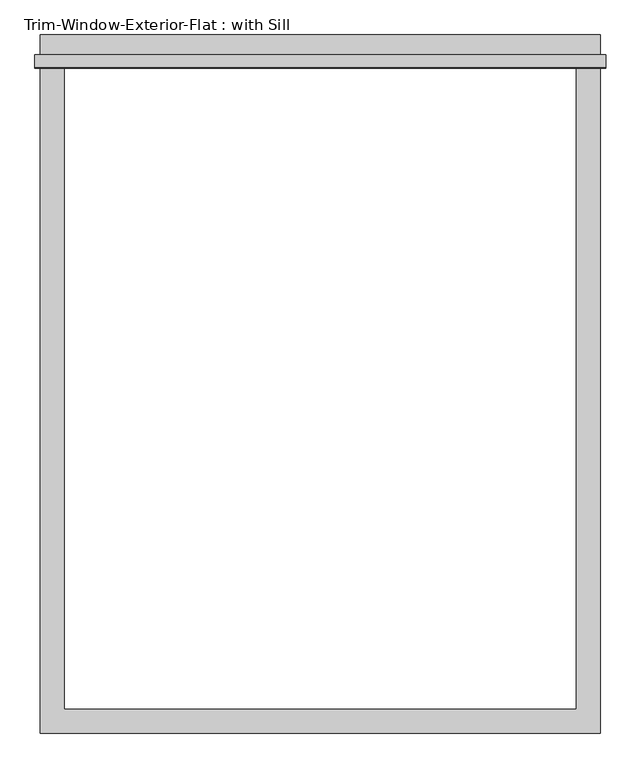
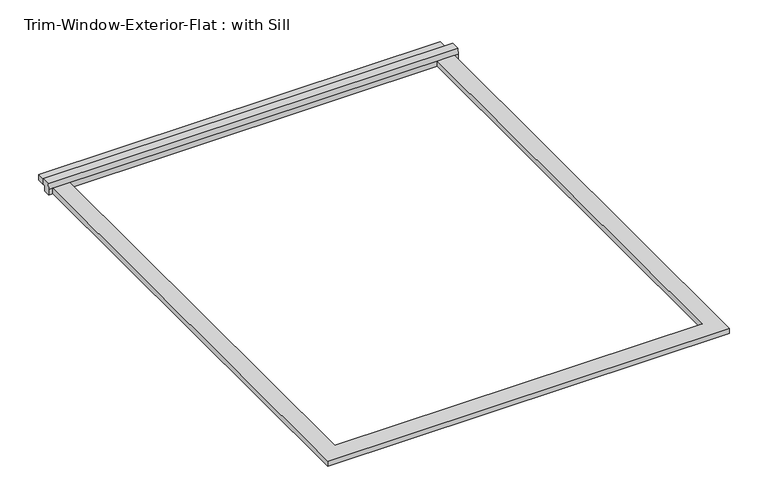
"""IFC4 building model written with IfcOpenShell, lengths in millimetres: proxy geometry, Trim-Window-Exterior-Flat : with Sill."""

from ifc_helpers import new_model, si_unit, frame, origin, origin_with_axes, place, context, project, spatial, polyline, outline, extrude, source, transform, mapped, element, save


def trim_window_exterior_flat_with_sill_e3be2e48(model_context):
    return source(origin(), model_context, "Body", "SweptSolid", [
        extrude(outline(polyline([(666.75, 1546.1823709), (-666.75, 1546.1823709), (-666.75, 1603.3323709), (666.75, 1603.3323709), (666.75, 1546.1823709)])), origin_with_axes(), (0.0, 0.0, 1.0), 19.05),
        extrude(outline(polyline([(1555.75, 38.1), (1555.75, 19.05), (1546.1823709, 19.05), (1546.1823709, 0.0), (1524.0, 0.0), (1524.0, 19.05), (1526.4580645, 38.1), (1555.75, 38.1)])), frame((-679.45, 0.0, 0.0), z_axis=(1.0, 0.0, 0.0), x_axis=(0.0, 1.0, 0.0)), (0.0, 0.0, 1.0), 1358.9),
        extrude(outline(polyline([(-666.75, -57.15), (-666.75, 1524.0), (-609.6, 1524.0), (-609.6, 0.0), (609.6, 0.0), (609.6, 1524.0), (666.75, 1524.0), (666.75, -57.15), (-666.75, -57.15)])), origin_with_axes(), (0.0, 0.0, 1.0), 19.05),
    ])


if __name__ == "__main__":
    model = new_model("IFC4")
    model_context = context("Model", 3, world=origin())
    ifc_project = project(units=[si_unit("LENGTHUNIT", "METRE", prefix="MILLI")], contexts=[model_context])
    site = spatial("IfcSite", under=ifc_project)
    building = spatial("IfcBuilding", under=site)
    placement = place(None, origin())
    trim_window_exterior_flat_with_sill_shape = trim_window_exterior_flat_with_sill_e3be2e48(model_context)
    element("IfcBuildingElementProxy", 1, Name="Trim-Window-Exterior-Flat : with Sill", ObjectType="Trim-Window-Exterior-Flat : with Sill", at=placement, inside=building, context=model_context, shape_type="MappedRepresentation", body=[
        mapped(trim_window_exterior_flat_with_sill_shape, transform((0.0, 0.0, 0.0), x_axis=(1.0, 0.0, 0.0), y_axis=(0.0, 1.0, 0.0), z_axis=(0.0, 0.0, 1.0))),
    ])
    save(model, "model.ifc")

# Revit data of these elements
# Type "Trim-Window-Exterior-Flat : with Sill"
#   Trim Width = 0' - 2 1/4"
#   Trim Thickness_Picture Frame = 0' - 1 1/4"
#   Trim Thickness_with Sill = 0' - 0 3/4"
#   Sill Thickness = 0' - 1 1/4"
#   Opening Width [instance default] = 2' - 0"
#   Opening Height [instance default] = 3' - 0"
#   Default Elevation = 4' - 0"
#   Sill = yes
#   Picture Frame = no
#   Trim Material [instance default] = none
# Element 1 (IfcBuildingElementProxy, "Trim-Window-Exterior-Flat : with Sill")
#   Opening Width = 4' - 0"
#   Opening Height = 5' - 0"
#   Trim Material = Clad - White
#   Materials on its faces: "Clad - White"
# Materials
#   "Clad - White": class "Wood", colour RGB 242 242 238, transparency 0, Cost = 0
